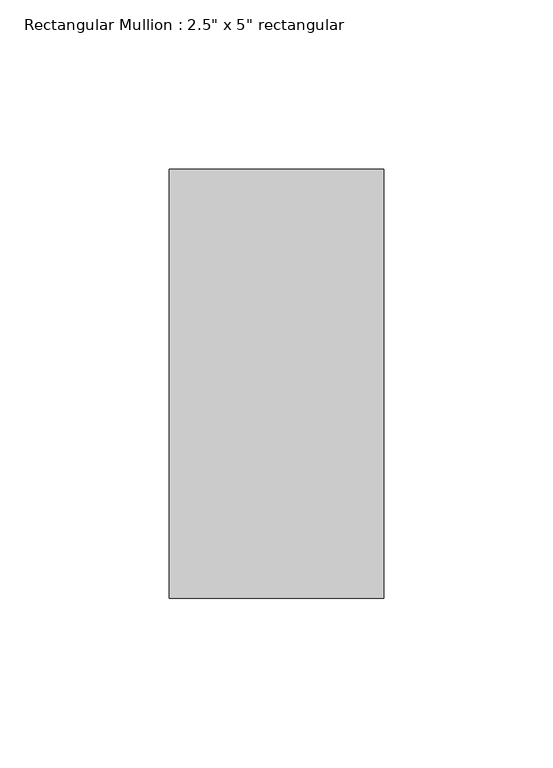
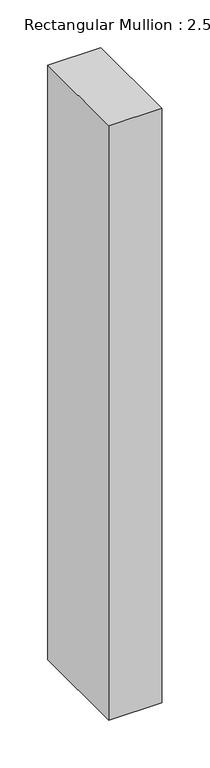
"""IFC4 building model written with IfcOpenShell, lengths in millimetres: member geometry."""

from ifc_helpers import new_model, si_unit, frame, origin, place, context, project, spatial, polyline, outline, extrude, source, transform, mapped, element, save


def member_a6ee1c2c(model_context):
    return source(origin(), model_context, "Body", "SweptSolid", [
        extrude(outline(polyline([(0.0, 63.5), (0.0, -63.5), (-63.5, -63.5), (-63.5, 63.5), (0.0, 63.5)])), frame((0.0, 0.0, -756.3361093), z_axis=(0.0, 0.0, 1.0), x_axis=(1.0, 0.0, 0.0)), (0.0, 0.0, 1.0), 756.3361093),
    ])


if __name__ == "__main__":
    model = new_model("IFC4")
    model_context = context("Model", 3, world=origin())
    ifc_project = project(units=[si_unit("LENGTHUNIT", "METRE", prefix="MILLI")], contexts=[model_context])
    site = spatial("IfcSite", under=ifc_project)
    building = spatial("IfcBuilding", under=site)
    placement = place(None, origin())
    member_shape = member_a6ee1c2c(model_context)
    element("IfcMember", 1, ObjectType="Rectangular Mullion : 2.5\" x 5\" rectangular", at=placement, inside=building, context=model_context, shape_type="MappedRepresentation", body=[
        mapped(member_shape, transform((0.0, 0.0, 0.0), x_axis=(1.0, 0.0, 0.0), y_axis=(0.0, 1.0, 0.0), z_axis=(0.0, 0.0, 1.0))),
    ])
    save(model, "model.ifc")

# Revit data of these elements
# Type "Rectangular Mullion : 2.5\" x 5\" rectangular"
#   built-in parameter 1007304 = 0.416667 (stored number, unit not read)
#   built-in parameter 1007301 = 0.104167 (stored number, unit not read)
#   built-in parameter 1007300 = 0.104167 (stored number, unit not read)
# Element 1 (IfcMember, "Rectangular Mullion : 2.5\" x 5\" rectangular")
#   Materials on its faces: "Aluminum"
# Materials
#   "Aluminum": class "Metal", colour RGB 247 247 247, transparency 0, Description = "Aluminum 6061", Cost = 0
